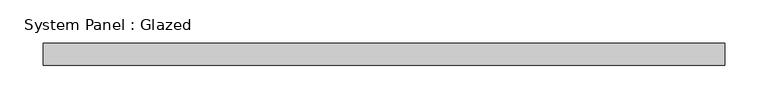
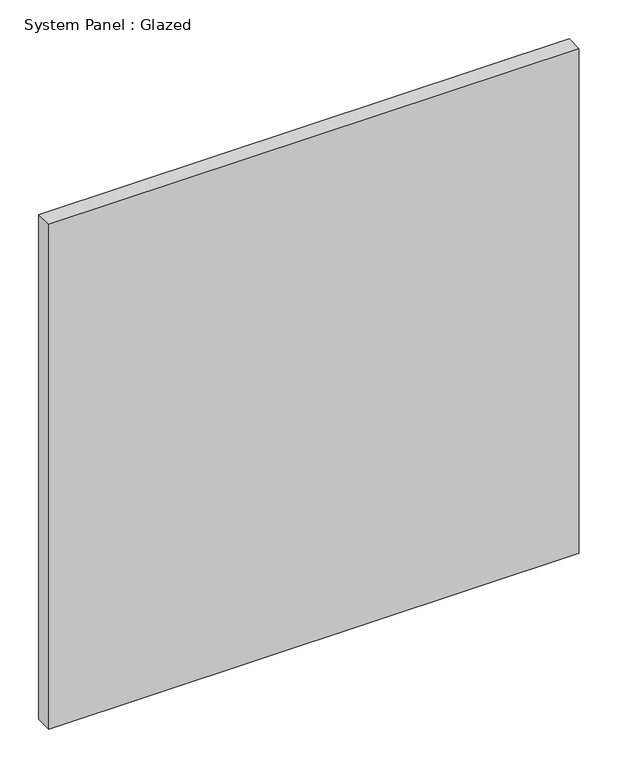
"""IFC4 building model written with IfcOpenShell, lengths in millimetres: plate geometry, System Panel : Glazed."""

from ifc_helpers import new_model, si_unit, origin, origin_with_axes, place, context, project, spatial, polyline, outline, extrude, source, transform, mapped, element, save


def system_panel_glazed_1e360deb(model_context):
    return source(origin(), model_context, "Body", "SweptSolid", [
        extrude(outline(polyline([(393.7, 19.05), (-393.7, 19.05), (-393.7, 44.45), (393.7, 44.45), (393.7, 19.05)])), origin_with_axes(), (0.0, 0.0, 1.0), 791.7415583),
    ])


if __name__ == "__main__":
    model = new_model("IFC4")
    model_context = context("Model", 3, world=origin())
    ifc_project = project(units=[si_unit("LENGTHUNIT", "METRE", prefix="MILLI")], contexts=[model_context])
    site = spatial("IfcSite", under=ifc_project)
    building = spatial("IfcBuilding", under=site)
    placement = place(None, origin())
    system_panel_glazed_shape = system_panel_glazed_1e360deb(model_context)
    element("IfcPlate", 1, ObjectType="System Panel : Glazed", at=placement, inside=building, context=model_context, shape_type="MappedRepresentation", body=[
        mapped(system_panel_glazed_shape, transform((0.0, 0.0, 0.0), x_axis=(1.0, 0.0, 0.0), y_axis=(0.0, 1.0, 0.0), z_axis=(0.0, 0.0, 1.0))),
    ])
    save(model, "model.ifc")

# Revit data of these elements
# Type "System Panel : Glazed"
#   Construction Type Id = "GSP4R"
#   Analytic Construction = "1/8 in Pilkington single glazing"
#   Visual Light Transmittance = 0.9
#   Solar Heat Gain Coefficient = 0.86
#   Heat Transfer Coefficient (U) = 1.18115 BTU/(h·ft²·°F)
#   Define Thermal Properties by = 1
# Element 1 (IfcPlate, "System Panel : Glazed")
#   Materials on its faces: "Glass"
# Materials
#   "Glass": class "Glass", colour RGB 0 128 192, transparency 0.75, Description = "Soda Lime Glass", Cost = 0
